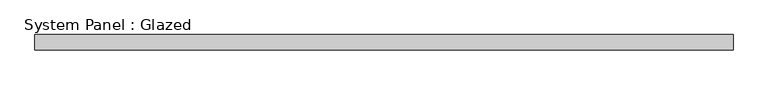
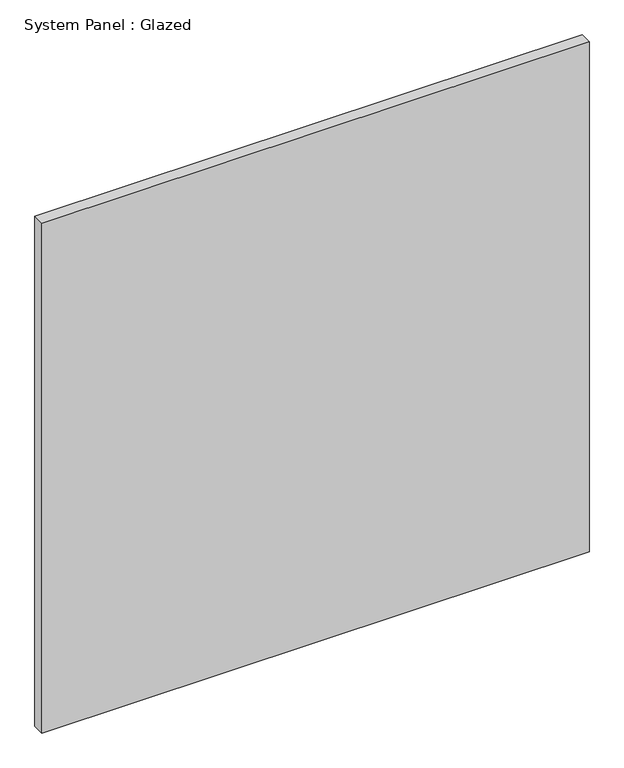
"""IFC4 building model written with IfcOpenShell, lengths in millimetres: plate geometry, System Panel : Glazed."""

from ifc_helpers import new_model, si_unit, origin, origin_with_axes, place, context, project, spatial, polyline, outline, extrude, source, transform, mapped, element, save


def system_panel_glazed_49652e9e(model_context):
    return source(origin(), model_context, "Body", "SweptSolid", [
        extrude(outline(polyline([(576.8975001, 19.05), (-576.8975001, 19.05), (-576.8975001, 44.45), (576.8975001, 44.45), (576.8975001, 19.05)])), origin_with_axes(), (0.0, 0.0, 1.0), 1137.1384615),
    ])


if __name__ == "__main__":
    model = new_model("IFC4")
    model_context = context("Model", 3, world=origin())
    ifc_project = project(units=[si_unit("LENGTHUNIT", "METRE", prefix="MILLI")], contexts=[model_context])
    site = spatial("IfcSite", under=ifc_project)
    building = spatial("IfcBuilding", under=site)
    placement = place(None, origin())
    system_panel_glazed_shape = system_panel_glazed_49652e9e(model_context)
    element("IfcPlate", 1, ObjectType="System Panel : Glazed", at=placement, inside=building, context=model_context, shape_type="MappedRepresentation", body=[
        mapped(system_panel_glazed_shape, transform((0.0, 0.0, 0.0), x_axis=(1.0, 0.0, 0.0), y_axis=(0.0, 1.0, 0.0), z_axis=(0.0, 0.0, 1.0))),
    ])
    save(model, "model.ifc")

# Revit data of these elements
# Type "System Panel : Glazed"
#   Construction Type Id = "GSP4R"
#   Analytic Construction = "1/8 in Pilkington single glazing"
#   Visual Light Transmittance = 0.9
#   Solar Heat Gain Coefficient = 0.86
#   Heat Transfer Coefficient (U) = 1.18115 BTU/(h·ft²·°F)
#   Define Thermal Properties by = 1
# Element 1 (IfcPlate, "System Panel : Glazed")
#   Materials on its faces: "Glass"
# Materials
#   "Glass": class "Glass", colour RGB 0 128 192, transparency 0.75, Description = "Soda Lime Glass", Cost = 0
